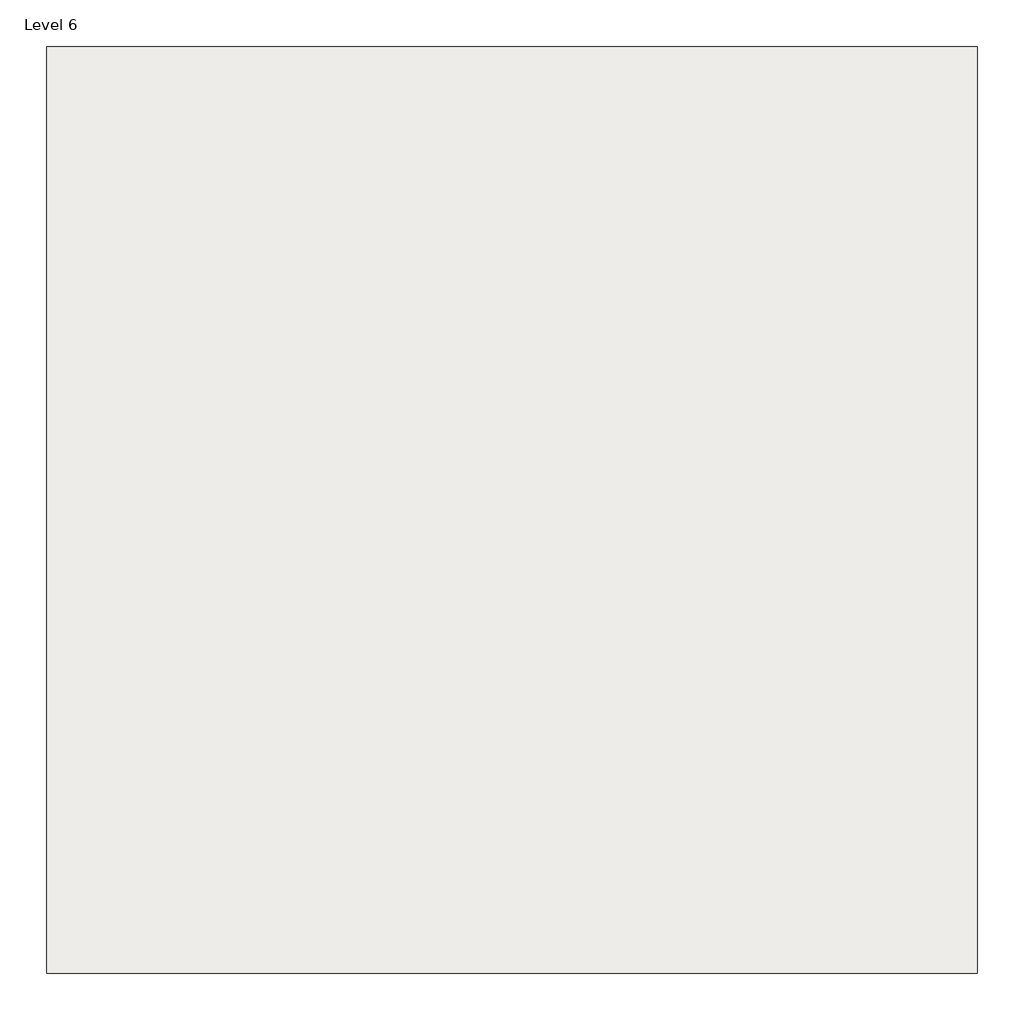
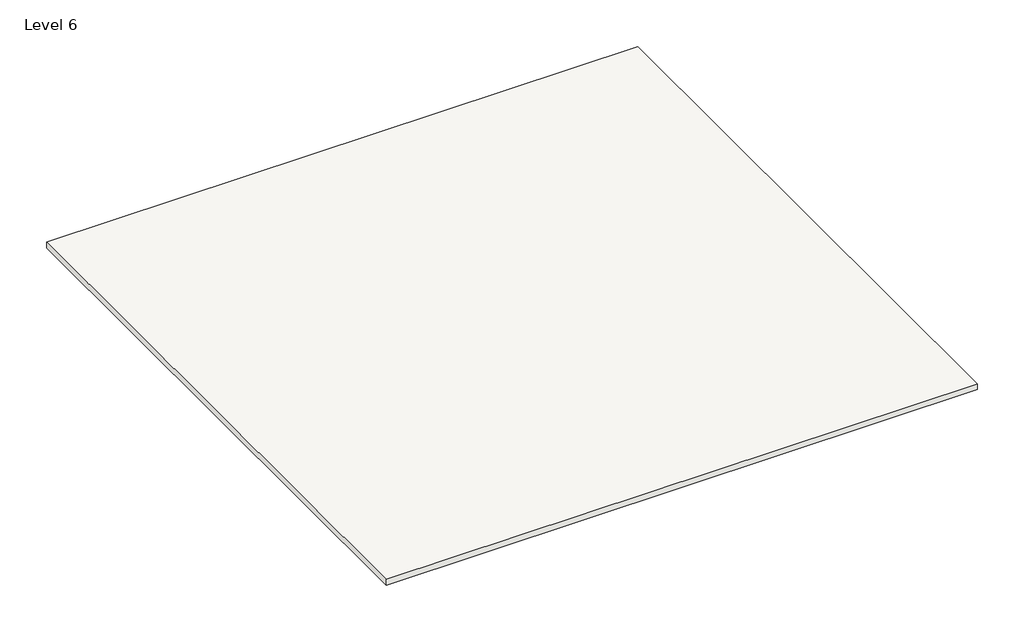
# One storey: 1 roof.
"""IFC4 building model written with IfcOpenShell, lengths in millimetres."""

from ifc_helpers import new_model, si_unit, frame, origin, place, context, project, spatial, polyline, outline, extrude, element, save

model = new_model("IFC4")

# Units and contexts
model_context = context("Model", 3, world=origin())
ifc_project = project(units=[si_unit("LENGTHUNIT", "METRE", prefix="MILLI")], contexts=[model_context])

# Site, building, storey
site = spatial("IfcSite", under=ifc_project)
building = spatial("IfcBuilding", under=site)
storey = spatial("IfcBuildingStorey", under=building, Name="Level 6", Elevation=9601.2)

# Roof
placement = place(None, origin())
element("IfcRoof", 1, ObjectType="Generic - 9\"", at=placement, inside=storey, context=model_context, shape_type="SweptSolid", body=[
    extrude(outline(polyline([(-8934.7629849, 17755.0995758), (12604.4370151, 17755.0995758), (12604.4370151, -3682.5004242), (-8934.7629849, -3682.5004242), (-8934.7629849, 17755.0995758)])), frame((0.0, 0.0, 9601.2), z_axis=(0.0, 0.0, 1.0), x_axis=(1.0, 0.0, 0.0)), (0.0, 0.0, 1.0), 228.6),
])

save(model, "model.ifc")

# Revit data of these elements
# Type "Generic - 9\""
#   Assembly Code = "B1020"
#   Layers, outside or top first: 0' - 9" no material (function 1)
# Element 1 (IfcRoof, "Generic - 9\"")
#   built-in parameter 1001705 = 32.25 (stored number, unit not read)
#   built-in parameter 1001710 = 33615
#   Phase Created = New Construction
#   Materials on its faces: "Default Roof"
# Materials
#   "Default Roof": colour RGB 88 101 114, transparency 0
